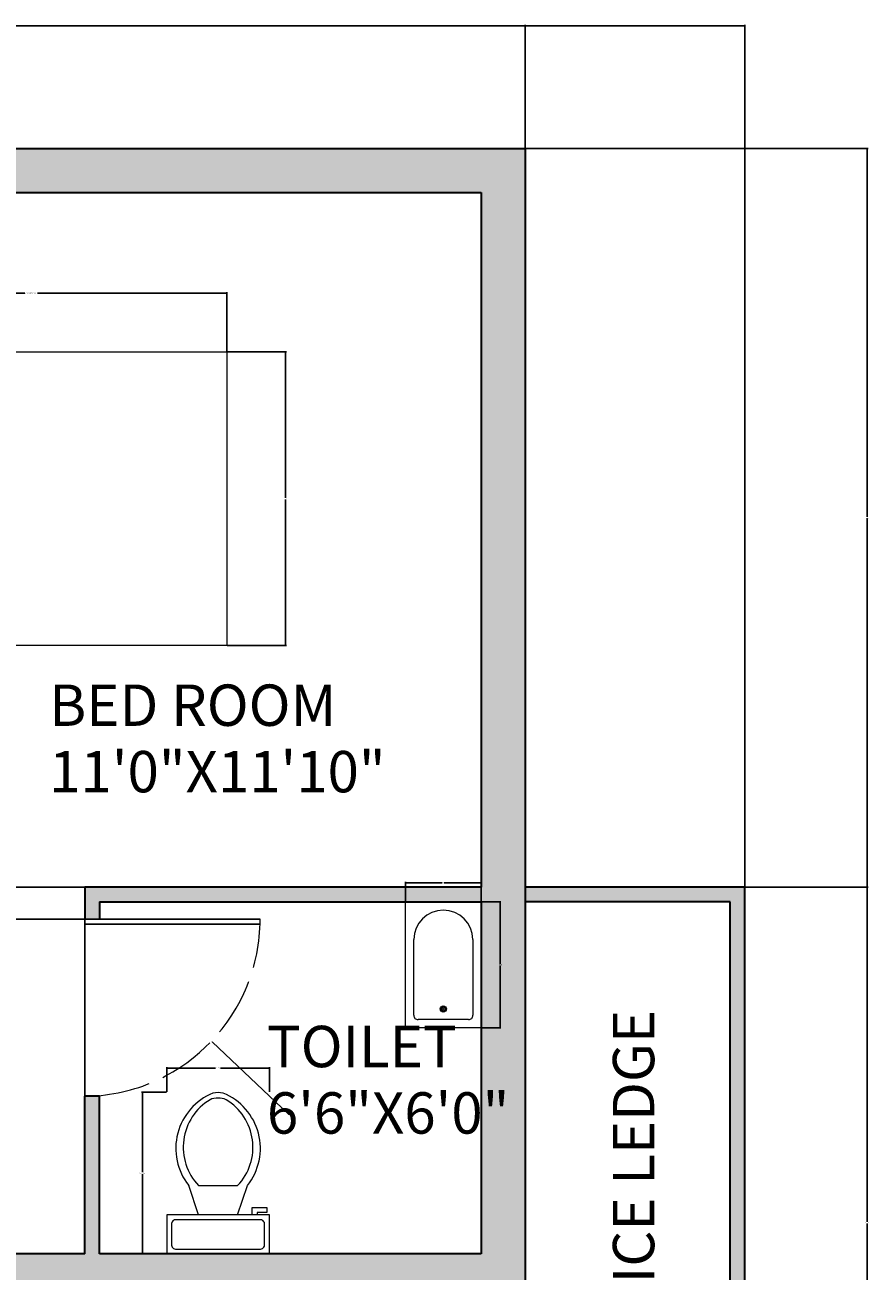
# Model space of a CAD drawing. Units: inches. Extents: x -12 to 539, y -477 to 51.
# Tile 6 of 6: x 367 to 539, y -203 to 51. Entities that reach past the tile are written whole.
import ezdxf

# ---------------------------------------------------------------- set-up
doc = ezdxf.new("R2010")
doc.units = ezdxf.units.IN
doc.header["$MEASUREMENT"] = 0
doc.linetypes.add('ACAD_ISO02W100', pattern=[15, 12, -3])
for name, color, linetype, lineweight in [('A-ANNO-DIMS', 2, 'Continuous', 18), ('A-AREA-IDEN', 7, 'Continuous', 18), ('A-DOOR', 4, 'Continuous', 25), ('A-DOOR-SWNG', 4, 'ACAD_ISO02W100', 13), ('A-FLOR-FIXT', 9, 'Continuous', 18), ('A-FURN', 8, 'Continuous', 18), ('A-WALL', 7, 'Continuous', 35)]:
    doc.layers.add(name, color=color, linetype=linetype, lineweight=lineweight)
doc.layers.add('A-WALL-PATT', color=252, linetype='Continuous', lineweight=13, true_color=0x939598)
doc.styles.get("Standard").update_dxf_attribs({"font": 'arial.ttf'})
doc.dimstyles.get("Standard").update_dxf_attribs({"dimtxt": 0.18, "dimasz": 0.18, "dimexe": 0.18, "dimexo": 0.0625, "dimgap": 0.09, "dimtad": 0, "dimtih": 1, "dimtoh": 1, "dimdec": 0, "dimzin": 0, "dimdsep": 46, "dimlunit": 3, "dimtxsty": 'Standard', "dimcen": 0.09, "dimadec": 0, "dimazin": 0, "dimtfac": 1, "dimtdec": 0, "dimtofl": 0, "dimtmove": 0, "dimatfit": 3, "dimfxl": 1, "dimtolj": 1, "dimtzin": 0, "dimarcsym": 0})

# ---------------------------------------------------------------- blocks, each defined once
blk = doc.blocks.new('Toilet - top')
for p, q in [((9.5, -6), (9.5, -2)), ((-10, -8.5), (-8, -8.5)), ((-10, -9.5), (-10, -8.5)), ((-7, -9.5), (-10, -9.5)), ((-8, -8.5), (-8, -8)), ((-7, -8), (-7, -9.5)), ((-4, -8), (-6, -14)), ((4, -8), (6, -14)), ((4, -14), (-4, -14))]:
    blk.add_line(p, q)
blk.add_lwpolyline([(10.5, -8), (10.5, 0), (-10.5, 0), (-10.5, -8)], close=True)
for points in [[(-9.5, -2), (-9.5, -6)], [(8.5, -1), (-8.5, -1)], [(-8.5, -7), (8.5, -7)]]:
    blk.add_lwpolyline(points)
for centre, radius, start, end in [((-8.62, -1.88), 0.884, 81.8699, 188.1301), ((8.62, -1.88), 0.884, 351.8699, 98.1301), ((-8.62, -6.12), 0.884, 171.8699, 278.1301), ((8.62, -6.12), 0.884, 261.8699, 8.1301), ((3.52, -21.58), 12.17, 141.4691, 247.9714), ((4.2, -21.82), 11.33, 136.3677, 238.9468), ((-3.52, -21.58), 12.17, 292.0284, 38.5307), ((-4.2, -21.82), 11.33, 301.053, 43.6321), ((0, -27.88), 4, 245.7318, 294.2682), ((0, -29), 4, 254.8605, 285.1395)]:
    blk.add_arc(centre, radius, start, end)
blk = doc.blocks.new('Bath Tub - 26 x 60 in.')
for p, q in [((9, -17), (9, -19)), ((8, -18), (10, -18))]:
    blk.add_line(p, q)
blk.add_lwpolyline([(0, -36), (0, 0), (60, 0), (60, -36)], close=True)
for points in [[(6, -4), (42, -4)], [(4, -30), (4, -6)], [(42, -32), (6, -32)]]:
    blk.add_lwpolyline(points)
for radius in [1.5, 1]:
    blk.add_circle((9, -18), radius)
for centre, radius, start, end in [((5.75, -5.75), 1.77, 81.8699, 188.1301), ((42, -18), 14, 270, 90), ((5.75, -30.25), 1.77, 171.8699, 278.1301)]:
    blk.add_arc(centre, radius, start, end)
blk = doc.blocks.new('Bed - Queen')
for p, q in [((0, -80.00003), (0, 0)), ((0, 0), (59.99999, 0)), ((59.99999, 0), (59.99999, -80.00003)), ((7.99999, -1.2), (28.79998, -1.2)), ((7.99999, -14.4), (7.99999, -1.2)), ((28.79998, -1.2), (28.79998, -14.4)), ((31.19999, -1.2), (51.99999, -1.2)), ((31.19999, -14.4), (31.19999, -1.2)), ((51.99999, -1.2), (51.99999, -16.4)), ((0, -14.4), (44.8, -14.4)), ((59.99999, -29.6), (44.8, -14.4)), ((44.8, -14.4), (44.8, -29.6)), ((44.8, -16.8), (0, -16.8)), ((51.99999, -16.4), (46.79936, -16.4)), ((44.8, -29.6), (59.99999, -29.6)), ((59.99999, -80.00003), (0, -80.00003))]:
    blk.add_line(p, q)
blk = doc.blocks.new('*D9')
at = {"layer": 'A-ANNO-DIMS', "color": 0, "lineweight": -2, "transparency": 16777216}
for p, q in [((328.1, -15.53), (328.1, -3.41)), ((328.28, -3.59), (366.8, -3.59)), ((407.92, -3.59), (369.41, -3.59)), ((408.1, -15.53), (408.1, -3.41))]:
    blk.add_line(p, q, dxfattribs=at)
at = {"layer": 'A-ANNO-DIMS', "color": 0, "transparency": 16777216}
for points in [[(328.28, -3.56), (328.28, -3.62), (328.1, -3.59)], [(407.92, -3.56), (407.92, -3.62), (408.1, -3.59)]]:
    blk.add_solid(points, dxfattribs=at)
at = {"layer": 'Defpoints', "color": 0, "transparency": 16777216}
for p in [(328.1, -3.59), (328.1, -15.59), (408.1, -15.59)]:
    blk.add_point(p, dxfattribs=at)
at = {"layer": 'A-ANNO-DIMS', "color": 0, "transparency": 16777216, "insert": (368.1, -3.59), "char_height": 0.18, "attachment_point": 5}
blk.add_mtext('\\A1;QUEEN BED 80 TYP.', dxfattribs=at)
blk = doc.blocks.new('*D10')
at = {"layer": 'A-ANNO-DIMS', "color": 0, "lineweight": -2, "transparency": 16777216}
for p, q in [((408.17, -15.59), (420.28, -15.59)), ((420.1, -15.77), (420.1, -45.41)), ((420.1, -75.41), (420.1, -45.77)), ((408.17, -75.59), (420.28, -75.59))]:
    blk.add_line(p, q, dxfattribs=at)
at = {"layer": 'A-ANNO-DIMS', "color": 0, "transparency": 16777216}
for points in [[(420.07, -15.77), (420.13, -15.77), (420.1, -15.59)], [(420.07, -75.41), (420.13, -75.41), (420.1, -75.59)]]:
    blk.add_solid(points, dxfattribs=at)
at = {"layer": 'Defpoints', "color": 0, "transparency": 16777216}
for p in [(408.1, -15.59), (420.1, -15.59), (408.1, -75.59)]:
    blk.add_point(p, dxfattribs=at)
at = {"layer": 'A-ANNO-DIMS', "color": 0, "transparency": 16777216, "insert": (420.1, -45.59), "char_height": 0.18, "attachment_point": 5}
blk.add_mtext('\\A1;60 TYP.', dxfattribs=at)
blk = doc.blocks.new('*D23')
at = {"layer": 'A-ANNO-DIMS', "color": 0, "lineweight": -2, "transparency": 16777216}
for p, q in [((460.17, -127.99), (464.15, -127.99)), ((463.97, -128.17), (463.97, -140.7)), ((463.97, -153.59), (463.97, -141.06)), ((460.17, -153.77), (464.15, -153.77))]:
    blk.add_line(p, q, dxfattribs=at)
at = {"layer": 'A-ANNO-DIMS', "color": 0, "transparency": 16777216}
for points in [[(463.94, -128.17), (464, -128.17), (463.97, -127.99)], [(463.94, -153.59), (464, -153.59), (463.97, -153.77)]]:
    blk.add_solid(points, dxfattribs=at)
at = {"layer": 'Defpoints', "color": 0, "transparency": 16777216}
for p in [(460.1, -127.99), (463.97, -127.99), (460.1, -153.77)]:
    blk.add_point(p, dxfattribs=at)
at = {"layer": 'A-ANNO-DIMS', "color": 0, "transparency": 16777216, "insert": (463.97, -140.88), "char_height": 0.18, "attachment_point": 5}
blk.add_mtext('\\A1;TUB 26', dxfattribs=at)
blk = doc.blocks.new('*D24')
at = {"layer": 'A-ANNO-DIMS', "color": 0, "lineweight": -2, "transparency": 16777216}
for p, q in [((444.63, -127.93), (444.63, -123.94)), ((444.81, -124.12), (452.16, -124.12)), ((459.92, -124.12), (452.58, -124.12)), ((460.1, -127.93), (460.1, -123.94))]:
    blk.add_line(p, q, dxfattribs=at)
at = {"layer": 'A-ANNO-DIMS', "color": 0, "transparency": 16777216}
for points in [[(444.81, -124.09), (444.81, -124.15), (444.63, -124.12)], [(459.92, -124.09), (459.92, -124.15), (460.1, -124.12)]]:
    blk.add_solid(points, dxfattribs=at)
at = {"layer": 'Defpoints', "color": 0, "transparency": 16777216}
for p in [(444.63, -124.12), (444.63, -127.99), (460.1, -127.99)]:
    blk.add_point(p, dxfattribs=at)
at = {"layer": 'A-ANNO-DIMS', "color": 0, "transparency": 16777216, "insert": (452.37, -124.12), "char_height": 0.18, "attachment_point": 5}
blk.add_mtext('\\A1;15', dxfattribs=at)
blk = doc.blocks.new('*D25')
at = {"layer": 'A-ANNO-DIMS', "color": 0, "lineweight": -2, "transparency": 16777216}
for p, q in [((395.76, -166.94), (390.69, -166.94)), ((390.87, -167.12), (390.87, -183.28)), ((390.87, -199.81), (390.87, -183.65)), ((395.76, -199.99), (390.69, -199.99))]:
    blk.add_line(p, q, dxfattribs=at)
at = {"layer": 'A-ANNO-DIMS', "color": 0, "transparency": 16777216}
for points in [[(390.84, -167.12), (390.9, -167.12), (390.87, -166.94)], [(390.84, -199.81), (390.9, -199.81), (390.87, -199.99)]]:
    blk.add_solid(points, dxfattribs=at)
at = {"layer": 'Defpoints', "color": 0, "transparency": 16777216}
for p in [(395.82, -166.94), (390.87, -199.99), (395.82, -199.99)]:
    blk.add_point(p, dxfattribs=at)
at = {"layer": 'A-ANNO-DIMS', "color": 0, "transparency": 16777216, "insert": (390.87, -183.46), "char_height": 0.18, "attachment_point": 5}
blk.add_mtext('\\A1;WC 33 TYP.', dxfattribs=at)
blk = doc.blocks.new('*D26')
at = {"layer": 'A-ANNO-DIMS', "color": 0, "lineweight": -2, "transparency": 16777216}
for p, q in [((395.82, -166.88), (395.82, -161.8)), ((396, -161.98), (405.79, -161.98)), ((416.64, -161.98), (406.85, -161.98)), ((416.82, -166.88), (416.82, -161.8))]:
    blk.add_line(p, q, dxfattribs=at)
at = {"layer": 'A-ANNO-DIMS', "color": 0, "transparency": 16777216}
for points in [[(396, -161.95), (396, -162.01), (395.82, -161.98)], [(416.64, -161.95), (416.64, -162.01), (416.82, -161.98)]]:
    blk.add_solid(points, dxfattribs=at)
at = {"layer": 'Defpoints', "color": 0, "transparency": 16777216}
for p in [(395.82, -161.98), (395.82, -166.94), (416.82, -166.94)]:
    blk.add_point(p, dxfattribs=at)
at = {"layer": 'A-ANNO-DIMS', "color": 0, "transparency": 16777216, "insert": (406.32, -161.98), "char_height": 0.18, "attachment_point": 5}
blk.add_mtext('\\A1;21 TYP.', dxfattribs=at)
blk = doc.blocks.new('*D36')
at = {"layer": 'A-ANNO-DIMS', "color": 0, "lineweight": -2, "transparency": 16777216}
for p, q in [((469.1, -124.93), (469.1, 51.25)), ((469.28, 51.07), (491.15, 51.07)), ((513.81, 51.07), (491.94, 51.07)), ((513.99, -124.93), (513.99, 51.25))]:
    blk.add_line(p, q, dxfattribs=at)
at = {"layer": 'A-ANNO-DIMS', "color": 0, "transparency": 16777216}
for points in [[(469.28, 51.1), (469.28, 51.04), (469.1, 51.07)], [(513.81, 51.1), (513.81, 51.04), (513.99, 51.07)]]:
    blk.add_solid(points, dxfattribs=at)
at = {"layer": 'Defpoints', "color": 0, "transparency": 16777216}
for p in [(513.99, 51.07), (469.1, -124.99), (513.99, -124.99)]:
    blk.add_point(p, dxfattribs=at)
at = {"layer": 'A-ANNO-DIMS', "color": 0, "transparency": 16777216, "insert": (491.54, 51.07), "char_height": 0.18, "attachment_point": 5}
blk.add_mtext('\\A1;44.88', dxfattribs=at)
blk = doc.blocks.new('*D37')
at = {"layer": 'A-ANNO-DIMS', "color": 0, "lineweight": -2, "transparency": 16777216}
for p, q in [((13.1, 26.07), (13.1, 51.25)), ((13.28, 51.07), (263.15, 51.07)), ((513.81, 51.07), (263.94, 51.07)), ((513.99, -124.93), (513.99, 51.25))]:
    blk.add_line(p, q, dxfattribs=at)
at = {"layer": 'A-ANNO-DIMS', "color": 0, "transparency": 16777216}
for points in [[(13.28, 51.1), (13.28, 51.04), (13.1, 51.07)], [(513.81, 51.1), (513.81, 51.04), (513.99, 51.07)]]:
    blk.add_solid(points, dxfattribs=at)
at = {"layer": 'Defpoints', "color": 0, "transparency": 16777216}
for p in [(513.99, 51.07), (13.1, 26.01), (513.99, -124.99)]:
    blk.add_point(p, dxfattribs=at)
at = {"layer": 'A-ANNO-DIMS', "color": 0, "transparency": 16777216, "insert": (263.54, 51.07), "char_height": 0.18, "attachment_point": 5}
blk.add_mtext('\\A1;500.9', dxfattribs=at)
blk = doc.blocks.new('*D39')
at = {"layer": 'A-ANNO-DIMS', "color": 0, "lineweight": -2, "transparency": 16777216}
for p, q in [((469.17, 26.01), (539.23, 26.01)), ((539.05, 25.83), (539.05, -49.31)), ((539.05, -124.81), (539.05, -49.67)), ((514.05, -124.99), (539.23, -124.99))]:
    blk.add_line(p, q, dxfattribs=at)
at = {"layer": 'A-ANNO-DIMS', "color": 0, "transparency": 16777216}
for points in [[(539.02, 25.83), (539.08, 25.83), (539.05, 26.01)], [(539.02, -124.81), (539.08, -124.81), (539.05, -124.99)]]:
    blk.add_solid(points, dxfattribs=at)
at = {"layer": 'Defpoints', "color": 0, "transparency": 16777216}
for p in [(469.1, 26.01), (513.99, -124.99), (539.05, -124.99)]:
    blk.add_point(p, dxfattribs=at)
at = {"layer": 'A-ANNO-DIMS', "color": 0, "transparency": 16777216, "insert": (539.05, -49.49), "char_height": 0.18, "attachment_point": 5}
blk.add_mtext('\\A1;151', dxfattribs=at)
blk = doc.blocks.new('*D40')
at = {"layer": 'A-ANNO-DIMS', "color": 0, "lineweight": -2, "transparency": 16777216}
for p, q in [((514.05, -124.99), (539.23, -124.99)), ((539.05, -125.17), (539.05, -193.41)), ((539.05, -262.02), (539.05, -193.78)), ((514.05, -262.2), (539.23, -262.2))]:
    blk.add_line(p, q, dxfattribs=at)
at = {"layer": 'A-ANNO-DIMS', "color": 0, "transparency": 16777216}
for points in [[(539.02, -125.17), (539.08, -125.17), (539.05, -124.99)], [(539.02, -262.02), (539.08, -262.02), (539.05, -262.2)]]:
    blk.add_solid(points, dxfattribs=at)
at = {"layer": 'Defpoints', "color": 0, "transparency": 16777216}
for p in [(513.99, -124.99), (513.99, -262.2), (539.05, -262.2)]:
    blk.add_point(p, dxfattribs=at)
at = {"layer": 'A-ANNO-DIMS', "color": 0, "transparency": 16777216, "insert": (539.05, -193.6), "char_height": 0.18, "attachment_point": 5}
blk.add_mtext('\\A1;137.22', dxfattribs=at)
blk = doc.blocks.new('*D53')
at = {"layer": 'A-ANNO-DIMS', "color": 0, "lineweight": -2, "transparency": 16777216}
for p, q in [((379.04, -124.99), (-12.14, -124.99)), ((-11.96, -125.17), (-11.96, -128.09)), ((-11.96, -131.38), (-11.96, -128.46)), ((379.04, -131.56), (-12.14, -131.56))]:
    blk.add_line(p, q, dxfattribs=at)
at = {"layer": 'A-ANNO-DIMS', "color": 0, "transparency": 16777216}
for points in [[(-11.99, -125.17), (-11.93, -125.17), (-11.96, -124.99)], [(-11.99, -131.38), (-11.93, -131.38), (-11.96, -131.56)]]:
    blk.add_solid(points, dxfattribs=at)
at = {"layer": 'Defpoints', "color": 0, "transparency": 16777216}
for p in [(379.1, -124.99), (-11.96, -131.56), (379.1, -131.56)]:
    blk.add_point(p, dxfattribs=at)
at = {"layer": 'A-ANNO-DIMS', "color": 0, "transparency": 16777216, "insert": (-11.96, -128.27), "char_height": 0.18, "attachment_point": 5}
blk.add_mtext('\\A1;6.575', dxfattribs=at)
blk = doc.blocks.new('*D62')
at = {"layer": 'A-ANNO-DIMS', "color": 0, "lineweight": -2, "transparency": 16777216}
for p, q in [((378.62, -131.56), (378.8, -131.56)), ((378.71, -131.65), (378.71, -131.47)), ((420.72, -171.44), (405.1, -156.61)), ((420.9, -171.44), (420.72, -171.44))]:
    blk.add_line(p, q, dxfattribs=at)
at = {"layer": 'A-ANNO-DIMS', "color": 0, "transparency": 16777216}
blk.add_solid([(405.12, -156.58), (405.08, -156.63), (404.97, -156.48)], dxfattribs=at)
at = {"layer": 'Defpoints', "color": 0, "transparency": 16777216}
for p in [(378.71, -131.56), (404.97, -156.48)]:
    blk.add_point(p, dxfattribs=at)
at = {"layer": 'A-ANNO-DIMS', "color": 0, "transparency": 16777216, "insert": (421.31, -171.44), "char_height": 0.18, "attachment_point": 5}
blk.add_mtext('\\A1;R36.2', dxfattribs=at)

msp = doc.modelspace()

# ---------------------------------------------------------------- hatches: boundary and pattern name
at = {"layer": 'A-WALL-PATT'}
h = msp.add_hatch(color=256, dxfattribs=at)
h.dxf.hatch_style = 1
h.paths.add_polyline_path([(267.143, 26.0124), (13.1031, 26.0124), (13.1031, -391.9876), (177.1031, -391.9876), (177.1031, -346.9876), (307.7315, -346.9876), (321.1031, -346.9876), (321.1031, -389.9876), (469.1031, -389.9876), (469.1031, 26.0124), (302.7142, 26.0124), (302.7142, 17.0124), (321.1031, 17.0124), (321.1031, -131.577, -0.04877504), (328.1031, -132.2621), (328.1031, 17.0124), (460.1031, 17.0124), (460.1031, -124.9876), (382.1031, -124.9876), (379.1031, -124.9876), (379.1031, -131.5624), (382.1031, -131.5624), (382.1031, -127.9876), (460.1031, -127.9876), (460.1031, -153.7747), (460.1031, -199.9876), (382.1031, -199.9876), (382.1031, -167.7132), (379.1031, -167.7132), (379.1031, -199.9876), (328.1031, -199.9876), (328.1031, -167.7132), (321.1031, -167.7132), (321.1031, -206.9876), (460.1031, -206.9876), (460.1031, -323.9876), (388.677, -323.9876, -0.02504709), (388.5266, -326.9876), (460.1031, -326.9876), (460.1031, -380.9876), (328.1031, -380.9876), (328.1031, -326.9876), (358.677, -326.9876), (358.677, -323.9876), (328.1031, -323.9876), (328.1031, -296.9562), (321.1031, -296.9562), (321.1031, -339.9876), (307.7315, -339.9876), (177.1031, -339.9876), (177.1031, -250.9876), (244.0259, -250.9876), (244.0259, -243.9876), (163.7315, -243.9876), (163.7315, -250.9876), (170.1031, -250.9876), (170.1031, -382.9876), (22.1031, -382.9876), (22.1031, -250.9876), (41.3871, -250.9876, -0.06888376), (40.8612, -243.9876), (22.1031, -243.9876), (22.1031, -183.9876), (118.1031, -183.9876), (118.1031, -243.9876), (71.6031, -243.9876), (71.6031, -250.9876), (128.4772, -250.9876, -0.04900189), (127.7315, -243.9876), (121.1031, -243.9876), (121.1031, -183.9876), (121.1031, -120.9876), (118.1031, -120.9876), (118.1031, -180.9876), (22.1031, -180.9876), (22.1031, -120.9876), (49.0045, -120.9876, -0.07000725), (46.9084, -111.9876), (46.1728, -111.9876), (22.1031, -111.9876), (22.1031, 17.0124), (170.1031, 17.0124), (170.1031, -120.9876), (177.1031, -120.9876), (177.1031, 17.0124), (268.2584, 17.0124, -0.0639977)])
h.paths.add_polyline_path([(513.9866, -124.9876), (469.1031, -124.9876), (469.1031, -127.9876), (510.9866, -127.9876), (510.9866, -259.2045), (469.1031, -259.2045), (469.1031, -262.2045), (513.9866, -262.2045)])
h.paths.add_polyline_path([(351.8833, -206.9876), (348.8833, -206.9876), (348.8833, -253.547), (328.1031, -253.547), (321.1031, -253.547), (321.1031, -256.547), (328.1031, -256.547), (351.8833, -256.547)], flags=17)
h.paths.add_polyline_path([(330.1031, -389.9876), (321.1031, -389.9876), (321.1031, -442.9876), (177.1031, -442.9876), (177.1031, -391.9876), (168.1031, -391.9876), (168.1031, -451.9876), (330.1031, -451.9876)])
h.paths.add_polyline_path([(414.1504, -177.6962), (465.5248, -177.6962), (465.5248, -164.7437), (414.1504, -164.7437)], flags=25)

# ---------------------------------------------------------------- linework, layer by layer
at = {"layer": 'A-DOOR'}
for p, q in [((379.1031, -167.7132), (379.1031, -131.5624)), ((379.1031, -131.5624), (414.9141, -131.5624)), ((379.1031, -132.5624), (414.9141, -132.5624))]:
    msp.add_line(p, q, dxfattribs=at)
at = {"layer": 'A-DOOR-SWNG'}
msp.add_arc((378.7139, -131.5624), 36.2002, 272.991421, 0, dxfattribs=at)
at = {"layer": 'A-WALL'}
for p, q in [((13.1031, 26.0124), (469.1031, 26.0124)), ((469.1031, 26.0124), (469.1031, -389.9876)), ((328.1031, 17.0124), (460.1031, 17.0124)), ((460.1031, 17.0124), (460.1031, -124.9876)), ((469.1031, 17.0124), (469.1031, -124.9876)), ((382.1031, -124.9876), (379.1031, -124.9876)), ((379.1031, -124.9876), (379.1031, -131.5624)), ((460.1031, -124.9876), (382.1031, -124.9876)), ((513.9866, -124.9876), (469.1031, -124.9876)), ((513.9866, -262.2045), (513.9866, -124.9876)), ((382.1031, -127.9876), (382.1031, -131.5624)), ((382.1031, -127.9876), (460.1031, -127.9876)), ((460.1031, -127.9876), (460.1031, -199.9876)), ((469.1031, -127.9876), (469.1031, -199.9876)), ((510.9866, -127.9876), (469.1031, -127.9876)), ((510.9866, -259.2045), (510.9866, -127.9876)), ((379.1031, -199.9876), (379.1031, -167.7132)), ((382.1031, -167.7132), (379.1031, -167.7132)), ((382.1031, -199.9876), (382.1031, -167.7132)), ((379.1031, -199.9876), (328.1031, -199.9876)), ((460.1031, -199.9876), (382.1031, -199.9876))]:
    msp.add_line(p, q, dxfattribs=at)

# ---------------------------------------------------------------- block references
at = {"layer": 'A-FLOR-FIXT', "xscale": 0.4297852123927119, "yscale": 0.4297852123927119, "zscale": 0.4297852123927119, "rotation": 90}
msp.add_blockref('Bath Tub - 26 x 60 in.', (444.6308, -153.7747), dxfattribs=at)
at = {"layer": 'A-FLOR-FIXT', "rotation": 180}
msp.add_blockref('Toilet - top', (406.3227, -199.9876), dxfattribs=at)
at = {"layer": 'A-FURN', "rotation": 90}
msp.add_blockref('Bed - Queen', (328.1031, -75.5882), dxfattribs=at)

# ---------------------------------------------------------------- texts
at = {"layer": 'A-AREA-IDEN'}
for s, height, p in [('BED ROOM ', 8.45618, (371.7948, -92.0395)), ('11\'0"X11\'10"', 8.456178, (371.7948, -105.6236)), ('TOILET', 8.45618, (416.3091, -161.8091)), ('6\'6"X6\'0"', 8.45618, (416.3091, -175.3933))]:
    msp.add_text(s, height=height, dxfattribs=at).set_placement(p)
msp.add_text('SERVICE LEDGE', height=8.456178, rotation=90, dxfattribs=at).set_placement((495.4985, -233.5965))

# ---------------------------------------------------------------- dimensions: what is measured, and where the dimension line sits
at = {"layer": 'A-ANNO-DIMS'}
for p1, override, picture, middle in [((13.1031, 26.0124), {"dimdec": 1, "dimlfac": 1, "dimrnd": 0, "dimzin": 0, "dimdsep": 46, "dimlunit": 2}, '*D37', (263.5448, 51.0724)), ((469.1031, -124.9876), {"dimdec": 2, "dimlfac": 1, "dimrnd": 0, "dimzin": 0, "dimdsep": 46, "dimlunit": 2}, '*D36', (491.5448, 51.0724))]:
    dim = msp.add_linear_dim(base=(513.9866, 51.0724), p1=p1, p2=(513.9866, -124.9876), dimstyle='Standard', override=override, dxfattribs=at)
    dim.commit()
    dim.dimension.update_dxf_attribs({"geometry": picture, "text_midpoint": middle})
for base, p1, p2, angle, override, picture, middle in [((539.0466, -124.9876), (469.1031, 26.0124), (513.9866, -124.9876), 90, {"dimdec": 0, "dimlfac": 1, "dimrnd": 0, "dimzin": 0, "dimdsep": 46, "dimlunit": 2}, '*D39', (539.0466, -49.4876)), ((444.6308, -124.1195), (460.1031, -127.9876), (444.6308, -127.9876), 180, {"dimdec": 0, "dimlfac": 1, "dimrnd": 0, "dimzin": 0, "dimdsep": 46, "dimlunit": 2}, '*D24', (452.3669, -124.1195)), ((-11.9569, -131.5624), (379.1031, -124.9876), (379.1031, -131.5624), 90, {"dimdec": 3, "dimlfac": 1, "dimrnd": 0, "dimzin": 0, "dimdsep": 46, "dimlunit": 2}, '*D53', (-11.9569, -128.275)), ((539.0466, -262.2045), (513.9866, -124.9876), (513.9866, -262.2045), 90, {"dimdec": 2, "dimlfac": 1, "dimrnd": 0, "dimzin": 0, "dimdsep": 46, "dimlunit": 2}, '*D40', (539.0466, -193.596))]:
    dim = msp.add_linear_dim(base=base, p1=p1, p2=p2, angle=angle, dimstyle='Standard', override=override, dxfattribs=at)
    dim.commit()
    dim.dimension.update_dxf_attribs({"geometry": picture, "text_midpoint": middle})
for base, p1, p2, angle, text, picture, middle in [((328.1031, -3.5882), (408.1031, -15.5882), (328.1031, -15.5882), 180, 'QUEEN BED <> TYP.', '*D9', (368.1031, -3.5882)), ((420.1031, -15.5882), (408.1031, -75.5882), (408.1031, -15.5882), 90, '<> TYP.', '*D10', (420.1031, -45.5882)), ((463.9711, -127.9876), (460.1031, -153.7747), (460.1031, -127.9876), 90, 'TUB <>', '*D23', (463.9711, -140.8811)), ((395.8227, -161.9844), (416.8227, -166.9413), (395.8227, -166.9413), 180, '<> TYP.', '*D26', (406.3227, -161.9844)), ((390.8657, -199.9876), (395.8227, -166.9413), (395.8227, -199.9876), 270, 'WC <> TYP.', '*D25', (390.8657, -183.4645))]:
    dim = msp.add_linear_dim(base=base, p1=p1, p2=p2, angle=angle, text=text, dimstyle='Standard', override={"dimdec": 0, "dimlfac": 1, "dimrnd": 0, "dimzin": 0, "dimdsep": 46, "dimlunit": 2}, dxfattribs=at)
    dim.commit()
    dim.dimension.update_dxf_attribs({"geometry": picture, "text_midpoint": middle})
dim = msp.add_radius_dim(center=(378.7139, -131.5624), mpoint=(404.9708, -156.4828), dimstyle='Standard', override={"dimdec": 1, "dimlfac": 1, "dimrnd": 0, "dimzin": 0, "dimdsep": 46, "dimlunit": 2}, dxfattribs=at)
dim.commit()
dim.dimension.update_dxf_attribs({"geometry": '*D62', "text_midpoint": (421.3139, -171.4351), "dimtype": 164})

doc.saveas('drawing.dxf')
